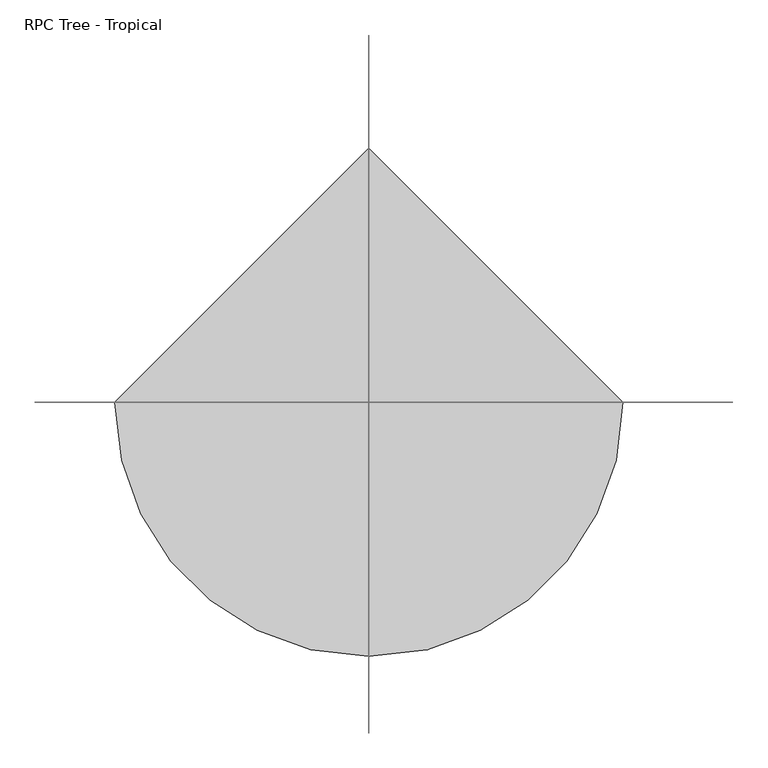
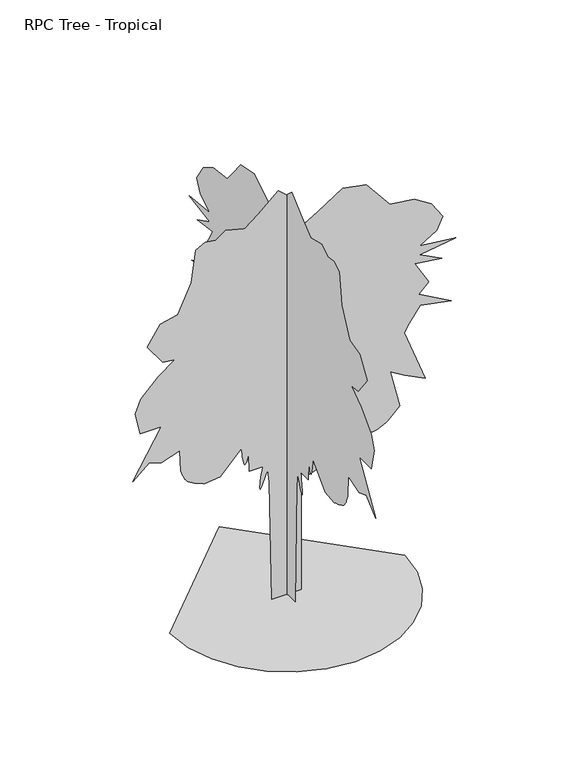
"""IFC4 building model written with IfcOpenShell, lengths in millimetres: geographic element geometry, RPC Tree - Tropical."""

from ifc_helpers import new_model, si_unit, origin, place, context, project, spatial, triangles, source, transform, mapped, element, save


def rpc_tree_tropical_d7a905c7(model_context):
    return source(origin(), model_context, "Body", "Tessellation", [
        triangles([(-0.2241189, -80.6803134, 0.0560704), (-0.2241181, -93.4507094, 708.3955685), (-0.2241176, -102.9729479, 784.5729681), (-0.2241171, -112.4304103, 759.6428038), (-0.2241163, -121.4992608, 736.1299221), (-0.2241158, -129.7908604, 715.4466642), (-0.2241156, -136.916343, 699.0127836), (-0.2241151, -142.4870876, 688.2406214), (-0.2241151, -146.1147278, 684.5474602), (-0.2241148, -147.4101338, 689.3505827), (-0.2241148, -146.9475984, 700.5392893), (-0.2241151, -145.6519381, 714.7252693), (-0.2241151, -143.662352, 731.4105881), (-0.2241153, -141.1175219, 750.0923693), (-0.2241156, -138.1563745, 770.2752216), (-0.2241156, -134.9173553, 791.458885), (-0.2241158, -131.5396545, 813.1404104), (-0.2241113, -207.7180624, 813.1404104), (-0.224111, -210.8920511, 914.7103008), (-0.2241108, -214.9636775, 900.580204), (-0.2241105, -218.9799477, 887.367057), (-0.2241105, -222.88496, 875.9827955), (-0.2241103, -226.6235945, 867.3493109), (-0.22411, -230.1402221, 862.3810095), (-0.2241097, -233.3789961, 861.9923704), (-0.2241095, -236.2847599, 867.1003435), (-0.2241095, -238.9129061, 876.4653969), (-0.2241092, -241.3744383, 887.9944897), (-0.2241092, -243.6972616, 901.3295042), (-0.224109, -245.9088635, 916.1097794), (-0.224109, -248.0373855, 931.9696398), (-0.2241087, -250.1102786, 948.5533659), (-0.2241087, -252.1552483, 965.4977531), (-0.2241016, -372.7715778, 838.5329012), (-0.2240963, -461.6464946, 829.010372), (-0.224095, -479.2563572, 835.8125004), (-0.224094, -496.4217339, 842.6147015), (-0.2240932, -512.6981023, 849.4168299), (-0.2240922, -527.64352, 856.2164148), (-0.2240914, -540.8134646, 863.0185432), (-0.2240907, -551.7608706, 869.8206717), (-0.2240902, -560.0413244, 876.6228727), (-0.2240899, -566.4726179, 884.1641275), (-0.2240897, -572.238436, 893.0389492), (-0.2240892, -577.4480018, 903.0236595), (-0.2240889, -582.2155887, 913.8974871), (-0.2240887, -586.6479126, 925.4367537), (-0.2240884, -590.8567037, 937.4204699), (-0.2240881, -594.9562717, 949.6252481), (-0.2240879, -601.3062839, 1073.4150759), (-0.2240815, -706.0511621, 1038.5001286), (-0.2240775, -775.8810568, 1063.8925467), (-0.2240719, -867.928418, 981.3677147), (-0.2240815, -706.0511621, 1254.3398609), (-0.2240744, -826.6659657, 1254.3398609), (-0.2240727, -855.233408, 1381.3021694), (-0.2240747, -823.4909414, 1460.6545933), (-0.2240805, -725.0961479, 1562.224411), (-0.2240861, -629.8712191, 1632.0567764), (-0.2240821, -699.7011137, 1641.5768349), (-0.224077, -785.4035133, 1759.0190849), (-0.2240813, -712.3985945, 1873.2865288), (-0.2240871, -614.0012575, 1895.5039227), (-0.2240917, -537.8238579, 2060.5586735), (-0.2240932, -512.4314034, 2247.8284927), (-0.2240963, -458.4714704, 2276.3959351), (-0.2240998, -398.1640686, 2266.8734058), (-0.2241034, -341.0291113, 2308.1358582), (-0.2241097, -233.1107712, 2279.5708866), (-0.2241143, -156.9326267, 2339.8783974), (-0.2241212, -42.6652782, 2438.2757343), (-0.2241265, 46.2093524, 2358.9233105), (-0.2241265, 46.2093524, 2263.6984543), (-0.2241298, 103.3427746, 2190.6960789), (-0.2241346, 182.6954255, 2235.1334827), (-0.224143, 322.3549604, 2327.1809166), (-0.2241509, 455.6672811, 2301.7884258), (-0.2241557, 538.1921494, 2200.2186081), (-0.2241588, 588.979638, 2136.7361458), (-0.2241672, 728.6394636, 2117.6910873), (-0.224173, 827.0368006, 2057.3837219), (-0.2241768, 890.5167194, 1958.986385), (-0.2241748, 855.6017721, 1889.1564903), (-0.2241689, 760.3793867, 1828.8489796), (-0.2241811, 963.5216383, 1806.6315857), (-0.2241689, 760.3793867, 1774.8890465), (-0.2241763, 884.1692144, 1711.4067295), (-0.2241674, 731.8118717, 1730.4516426), (-0.224172, 811.1642956, 1593.9668049), (-0.2241687, 754.0318817, 1540.0068718), (-0.2241796, 938.1291475, 1435.2621025), (-0.2241692, 763.5544109, 1470.1769772), (-0.2241654, 700.0719486, 1384.477121), (-0.2241636, 671.5045063, 1336.8647655), (-0.224171, 792.1193098, 1022.630167), (-0.2241639, 674.6795305, 1079.7650517), (-0.224159, 592.1520824, 1130.5500332), (-0.2241621, 646.1120155, 908.3627958), (-0.2241583, 579.4571451, 841.7079254), (-0.2241575, 566.5462689, 834.2758209), (-0.2241567, 553.721761, 827.1511105), (-0.224156, 541.0623593, 820.6359558), (-0.2241552, 528.6518887, 815.0378237), (-0.2241544, 516.5766809, 810.6613466), (-0.2241537, 504.9155105, 807.8089771), (-0.2241532, 493.7572526, 806.7929054), (-0.2241524, 482.6879065, 807.6260668), (-0.2241519, 471.2883479, 809.9577559), (-0.2241511, 459.6093733, 813.5392233), (-0.2241504, 447.7094456, 818.1188129), (-0.2241496, 435.6418682, 823.4503189), (-0.2241489, 423.4625244, 829.2796143), (-0.2241481, 411.2298409, 835.357877), (-0.2241481, 407.7779803, 839.4116993), (-0.2241478, 404.0213056, 843.2979446), (-0.2241476, 399.6524952, 846.8514341), (-0.2241471, 394.3692784, 849.9070616), (-0.2241468, 387.8643339, 852.2946339), (-0.2241463, 379.8302676, 853.8491175), (-0.2241458, 369.9674249, 854.4028627), (-0.224145, 357.1403735, 855.883659), (-0.224144, 340.8157522, 860.0289728), (-0.2241428, 321.5777186, 866.3967527), (-0.2241415, 300.0079778, 874.5400057), (-0.2241402, 276.6881621, 884.0168255), (-0.2241387, 252.2014664, 894.3800737), (-0.2241372, 227.1326114, 905.1877716), (-0.2241349, 185.8694142, 857.577887), (-0.2241349, 185.8694142, 778.2254631), (-0.2241362, 208.0876256, 702.0480635), (-0.2241316, 131.9097354, 676.6556454), (-0.2241288, 87.4725496, 800.4429296), (-0.2241293, 88.096376, 0.0), (-666.8181644, -2.5e-06, 0.2128606), (-649.2007078, -152.6793797, 0.2128611), (-599.0329851, -292.8908795, 0.2128626), (-520.3257617, -416.61723, 0.2128649), (-417.1023385, -519.8431603, 0.2128679), (-293.3760243, -598.5478403, 0.2128717), (-153.1642702, -648.715563, 0.2128758), (-0.4850755, -666.3330196, 0.2128804), (152.1942349, -648.715563, 0.2128849), (292.4057347, -598.5478403, 0.212889), (416.1320852, -519.8406169, 0.2128928), (519.3580155, -416.61723, 0.2128959), (598.0626955, -292.8908795, 0.2128981), (648.2304182, -152.6791254, 0.2128997), (665.8478748, 5.82e-05, 0.2129002), (-0.4851924, 666.3330196, 0.2128804), (-89.341994, 0.0001455, 0.1894216), (-102.11239, 0.0001057, 708.5276825), (-111.6346285, 9.96e-05, 784.7075529), (-121.0920909, 0.0001025, 759.7773886), (-130.1609414, 0.0001023, 736.2619635), (-138.4522867, 0.0001051, 715.581249), (-145.5777693, 0.000105, 699.144825), (-151.1487682, 0.0001048, 688.3726627), (-154.7761631, 0.0001075, 684.682045), (-156.0718144, 0.0001043, 689.4852402), (-155.6090338, 0.0001041, 700.6714033), (-154.3136187, 0.0001037, 714.8573833), (-152.3240326, 0.0001034, 731.5426294), (-149.7792025, 0.0001031, 750.2269541), (-146.8178008, 9.98e-05, 770.4098791), (-143.5790359, 9.95e-05, 791.590999), (-140.2013351, 9.92e-05, 813.2725245), (-216.3794887, 9.82e-05, 813.2725245), (-219.5534773, 9.2e-05, 914.8448856), (-223.6253582, 9.2e-05, 900.7147888), (-227.6413739, 9.5e-05, 887.4991711), (-231.5466406, 9.5e-05, 876.1173803), (-235.2852751, 9.49e-05, 867.4838957), (-238.8016665, 9.47e-05, 862.5131235), (-242.0406767, 9.44e-05, 862.1244844), (-244.9461861, 9.4e-05, 867.2324575), (-247.5745867, 9.35e-05, 876.5974382), (-250.0361189, 9.29e-05, 888.1290745), (-252.358706, 9.23e-05, 901.464089), (-254.5697811, 9.17e-05, 916.2418934), (-256.6983031, 9.1e-05, 932.1042246), (-258.7709418, 9.04e-05, 948.6854073), (-260.8156571, 8.97e-05, 965.6297945), (-381.4330041, 9.73e-05, 838.667486), (-470.3079208, 9.84e-05, 829.1450294), (-487.9177835, 9.66e-05, 835.9446144), (-505.0831601, 9.78e-05, 842.7467428), (-521.3595285, 9.61e-05, 849.5488712), (-536.3049462, 9.46e-05, 856.3510723), (-549.4748909, 9.61e-05, 863.1532007), (-560.4222968, 9.49e-05, 869.9527857), (-568.7027507, 9.4e-05, 876.7549141), (-575.1340442, 9.32e-05, 884.2962416), (-580.8998623, 9.24e-05, 893.1709906), (-586.109428, 9.17e-05, 903.1557735), (-590.8770149, 9.38e-05, 914.0295284), (-595.3093389, 9.31e-05, 925.568795), (-599.5181299, 9.23e-05, 937.5525839), (-603.617698, 9.16e-05, 949.759833), (-609.9677101, 8.15e-05, 1073.5496607), (-714.7125521, 8.49e-05, 1038.6347134), (-784.5424467, 8.37e-05, 1064.0272041), (-876.5898079, 8.96e-05, 981.4997561), (-714.7125521, 7.26e-05, 1254.4719749), (-835.3274282, 7.35e-05, 1254.4719749), (-863.8948706, 6.42e-05, 1381.4367542), (-832.152404, 5.89e-05, 1460.7891781), (-733.7575378, 5.3e-05, 1562.3589958), (-638.532609, 5.06e-05, 1632.1888905), (-708.3625763, 4.99e-05, 1641.7114197), (-794.0649759, 4.17e-05, 1759.1538151), (-721.0600571, 3.61e-05, 1873.4184975), (-622.6626474, 3.25e-05, 1895.6385075), (-546.4852841, 2.27e-05, 2060.6907875), (-521.0928297, 1.36e-05, 2247.9630775), (-467.1328966, 1.17e-05, 2276.5305199), (-406.8254949, 1.15e-05, 2267.0079906), (-349.6905375, 9.6e-06, 2308.270443), (-241.7724518, 1.13e-05, 2279.7030006), (-165.5940529, 7.6e-06, 2340.0103661), (-51.3267045, 3e-07, 2438.4078484), (37.5476695, 7.7e-06, 2359.0554245), (37.5476695, 1.34e-05, 2263.8330391), (94.6810849, 1.78e-05, 2190.8281929), (174.0337449, 1.48e-05, 2235.2655968), (313.6935342, 7e-06, 2327.3155014), (447.0058548, 1.09e-05, 2301.9230106), (529.5307231, 1.55e-05, 2200.3505768), (580.3182117, 1.9e-05, 2136.8682598), (719.978001, 2.04e-05, 2117.8258175), (818.3728672, 2.51e-05, 2057.515836), (881.8552568, 3.08e-05, 1959.1209698), (846.9403095, 3.56e-05, 1889.2910751), (751.7179241, 3.77e-05, 1828.9837097), (954.8601757, 3.9e-05, 1806.7636997), (751.7179241, 4.22e-05, 1775.0237766), (875.5077518, 4.35e-05, 1711.5413143), (723.1504818, 4.39e-05, 1730.5862274), (802.502833, 5.21e-05, 1594.0989189), (745.3704918, 5.45e-05, 1540.1416019), (929.4676849, 6.24e-05, 1435.3942165), (754.8929483, 6.03e-05, 1470.3117073), (691.4105587, 6.3e-05, 1384.609235), (662.8430437, 6.77e-05, 1336.9993504), (783.4579199, 8.5e-05, 1022.7647518), (666.0180679, 8.15e-05, 1079.8971657), (583.4906562, 7.85e-05, 1130.6820745), (637.4506256, 9.28e-05, 908.4973806), (570.7957189, 9.76e-05, 841.8399668), (557.8848427, 9.67e-05, 834.4104784), (545.0603348, 9.87e-05, 827.2831518), (532.4009331, 9.77e-05, 820.7706133), (519.9904624, 9.97e-05, 815.169865), (507.9152547, 9.88e-05, 810.7934607), (496.2540842, 9.78e-05, 807.9435619), (485.0932829, 9.98e-05, 806.9250195), (474.0264802, 9.87e-05, 807.7581808), (462.6269217, 9.77e-05, 810.0898699), (450.947947, 9.94e-05, 813.6712646), (439.0480193, 9.82e-05, 818.2534704), (426.980442, 9.7e-05, 823.5823603), (414.8010982, 9.86e-05, 829.4117283), (402.5684146, 9.74e-05, 835.4924618), (399.1165541, 9.69e-05, 839.5463568), (395.3598793, 9.65e-05, 843.4325294), (390.9910689, 9.6e-05, 846.9860189), (385.7078522, 9.54e-05, 850.0391029), (379.2029077, 9.48e-05, 852.4267479), (371.1688414, 9.69e-05, 853.9812315), (361.3059986, 9.6e-05, 854.5374475), (348.4789473, 9.48e-05, 856.0183165), (332.154326, 9.62e-05, 860.1635576), (312.9162924, 9.43e-05, 866.5288668), (291.3465516, 9.5e-05, 874.6721197), (268.0267359, 9.56e-05, 884.1488668), (243.5397858, 9.31e-05, 894.5146585), (218.4709308, 9.34e-05, 905.3224291), (177.2077336, 9.7e-05, 857.7099283), (177.2077336, 9.94e-05, 778.3575771), (199.4261993, 0.0001036, 702.1801775), (123.2483092, 0.0001063, 676.7876867), (78.8108599, 9.87e-05, 800.5775145), (79.4346863, 0.0001459, 0.1333563)], [[85, 84, 86], [53, 52, 54], [91, 90, 92], [87, 86, 88], [95, 94, 96], [96, 94, 97], [9, 8, 10], [52, 51, 54], [51, 50, 54], [1, 133, 2], [133, 132, 2], [2, 132, 3], [131, 130, 132], [130, 129, 132], [129, 128, 132], [18, 17, 19], [71, 70, 72], [72, 70, 73], [10, 8, 11], [8, 7, 11], [11, 7, 12], [7, 6, 12], [12, 6, 13], [6, 5, 13], [13, 5, 14], [5, 4, 14], [14, 4, 15], [4, 3, 15], [15, 3, 16], [16, 3, 17], [55, 54, 56], [89, 88, 90], [56, 54, 57], [57, 54, 58], [61, 60, 62], [62, 60, 63], [60, 59, 63], [25, 24, 26], [24, 23, 26], [26, 23, 27], [23, 22, 27], [27, 22, 28], [22, 21, 28], [28, 21, 29], [21, 20, 29], [29, 20, 30], [20, 19, 30], [30, 19, 31], [82, 81, 83], [83, 81, 84], [81, 80, 84], [80, 79, 84], [70, 69, 73], [98, 97, 99], [31, 19, 32], [99, 97, 100], [58, 54, 59], [100, 97, 101], [101, 97, 102], [102, 97, 103], [103, 97, 104], [104, 97, 105], [105, 97, 106], [106, 97, 107], [107, 97, 108], [108, 97, 109], [109, 97, 110], [110, 97, 111], [111, 97, 112], [112, 97, 113], [113, 97, 114], [114, 97, 115], [115, 97, 116], [116, 97, 117], [117, 97, 118], [118, 97, 119], [119, 97, 120], [120, 97, 121], [121, 97, 122], [122, 97, 123], [123, 97, 124], [124, 97, 125], [125, 97, 126], [126, 97, 127], [65, 64, 66], [66, 64, 67], [68, 67, 69], [67, 64, 69], [3, 132, 17], [73, 69, 74], [69, 64, 74], [64, 63, 74], [63, 59, 74], [17, 132, 19], [132, 128, 19], [128, 127, 19], [92, 90, 93], [76, 75, 77], [77, 75, 78], [78, 75, 79], [79, 75, 84], [75, 74, 84], [74, 59, 84], [84, 59, 86], [86, 59, 88], [88, 59, 90], [90, 59, 93], [93, 59, 94], [94, 59, 97], [97, 59, 127], [127, 59, 19], [32, 19, 33], [19, 59, 33], [59, 54, 33], [54, 50, 33], [33, 50, 34], [50, 49, 34], [34, 49, 35], [35, 49, 36], [36, 49, 37], [49, 48, 37], [37, 48, 38], [48, 47, 38], [38, 47, 39], [47, 46, 39], [39, 46, 40], [46, 45, 40], [45, 44, 40], [40, 44, 41], [44, 43, 41], [41, 43, 42], [148, 149, 134], [147, 148, 134], [147, 134, 135], [146, 147, 135], [146, 135, 136], [146, 136, 137], [145, 146, 137], [144, 145, 137], [144, 137, 138], [144, 138, 139], [144, 139, 140], [144, 140, 141], [144, 141, 142], [144, 142, 143], [233, 234, 235], [201, 202, 203], [239, 240, 241], [235, 236, 237], [243, 244, 245], [243, 245, 246], [157, 158, 159], [200, 201, 203], [199, 200, 203], [282, 150, 151], [281, 282, 151], [281, 151, 152], [279, 280, 281], [278, 279, 281], [277, 278, 281], [166, 167, 168], [219, 220, 221], [219, 221, 222], [157, 159, 160], [156, 157, 160], [156, 160, 161], [155, 156, 161], [155, 161, 162], [154, 155, 162], [154, 162, 163], [153, 154, 163], [153, 163, 164], [152, 153, 164], [152, 164, 165], [152, 165, 166], [203, 204, 205], [237, 238, 239], [203, 205, 206], [203, 206, 207], [209, 210, 211], [209, 211, 212], [208, 209, 212], [173, 174, 175], [172, 173, 175], [172, 175, 176], [171, 172, 176], [171, 176, 177], [170, 171, 177], [170, 177, 178], [169, 170, 178], [169, 178, 179], [168, 169, 179], [168, 179, 180], [230, 231, 232], [230, 232, 233], [229, 230, 233], [228, 229, 233], [218, 219, 222], [246, 247, 248], [168, 180, 181], [246, 248, 249], [203, 207, 208], [246, 249, 250], [246, 250, 251], [246, 251, 252], [246, 252, 253], [246, 253, 254], [246, 254, 255], [246, 255, 256], [246, 256, 257], [246, 257, 258], [246, 258, 259], [246, 259, 260], [246, 260, 261], [246, 261, 262], [246, 262, 263], [246, 263, 264], [246, 264, 265], [246, 265, 266], [246, 266, 267], [246, 267, 268], [246, 268, 269], [246, 269, 270], [246, 270, 271], [246, 271, 272], [246, 272, 273], [246, 273, 274], [246, 274, 275], [246, 275, 276], [213, 214, 215], [213, 215, 216], [216, 217, 218], [213, 216, 218], [281, 152, 166], [218, 222, 223], [213, 218, 223], [212, 213, 223], [208, 212, 223], [281, 166, 168], [277, 281, 168], [276, 277, 168], [239, 241, 242], [224, 225, 226], [224, 226, 227], [224, 227, 228], [224, 228, 233], [223, 224, 233], [208, 223, 233], [208, 233, 235], [208, 235, 237], [208, 237, 239], [208, 239, 242], [208, 242, 243], [208, 243, 246], [208, 246, 276], [208, 276, 168], [168, 181, 182], [208, 168, 182], [203, 208, 182], [199, 203, 182], [199, 182, 183], [198, 199, 183], [198, 183, 184], [198, 184, 185], [198, 185, 186], [197, 198, 186], [197, 186, 187], [196, 197, 187], [196, 187, 188], [195, 196, 188], [195, 188, 189], [194, 195, 189], [193, 194, 189], [193, 189, 190], [192, 193, 190], [192, 190, 191]], closed=False),
    ])


if __name__ == "__main__":
    model = new_model("IFC4")
    model_context = context("Model", 3, world=origin())
    ifc_project = project(units=[si_unit("LENGTHUNIT", "METRE", prefix="MILLI")], contexts=[model_context])
    site = spatial("IfcSite", under=ifc_project)
    building = spatial("IfcBuilding", under=site)
    placement = place(None, origin())
    rpc_tree_tropical_shape = rpc_tree_tropical_d7a905c7(model_context)
    element("IfcGeographicElement", 1, ObjectType="RPC Tree - Tropical", at=placement, inside=building, context=model_context, shape_type="MappedRepresentation", body=[
        mapped(rpc_tree_tropical_shape, transform((0.0, 0.0, 0.0), x_axis=(1.0, 0.0, 0.0), y_axis=(0.0, 1.0, 0.0), z_axis=(0.0, 0.0, 1.0))),
    ])
    save(model, "model.ifc")

# Revit data of these elements
# Type "RPC Tree - Tropical"
#   built-in parameter 1005198 = "{2, 15},{39, RPC-16-G2MF-J1Q0-CAN1-N000-ST1L-LVER-AU},{1, 0},{1, 0},{2, 13},{1, 8},{5, Color},{1, 0},{1, 0},{3, 0.8},{3, 0.8},{3, 0.8},{1, 8},{7, BBoxMin},{1, 0},{1, 0},{1, 0},{1, 0},{1, 0},{1, 8},{7, BBoxMax},{1, 0},{1, 0},{1, 0},{1, 0},{1, 0},{2, 11},{9, RPCTypeId},{1, 0},{1, 0},{39, RPC-16-G2MF-J1Q0-CAN1-N000-ST1L-LVER-AU},{1, 6},{14, RPCPlantHeight},{1, 0},{1, 0},{1, 8},{2, 11},{7, keyword},{1, 0},{1, 0},{35, :RPCs:Trees [Tropical]:Geometry:RPC},{2, 11},{8, category},{1, 0},{1, 0},{16, Trees [Tropical]},{2, 11},{12, LocalizedUID},{1, 0},{1, 0},{13, Windmill Palm},{2, 14},{6, Height},{1, 0},{1, 0},{1, 8},{1, 2},{16, Cast Reflections},{1, 0},{1, 0},{1, 0},{1, 2},{12, Cast Shadows},{1, 0},{1, 0},{1, 1},{1, 2},{9, Lock View},{1, 0},{1, 0},{1, 0},{1, 4},{5, ViewC},{1, 0},{1, 0},{1, 0},{21, assetlibrary_base.fbx},{1, 5},"
#   built-in parameter 1005195 = "RPC-16-G2MF-J1Q0-CAN1-N000-ST1L-LVER-AU"
#   Assembly Code = "G2050500"
#   Height = 8' - 0"
#   Plan Symbol = element 370751
#   Default Elevation = 0
